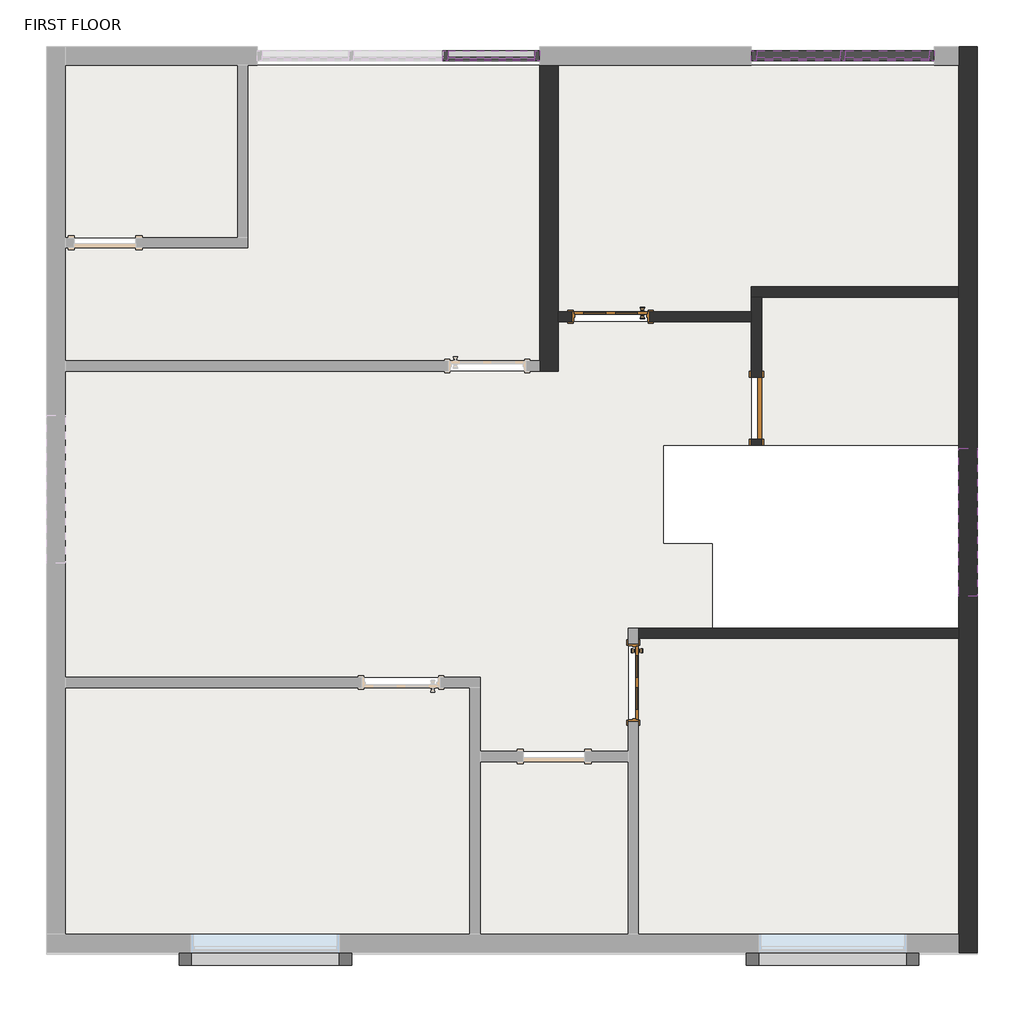
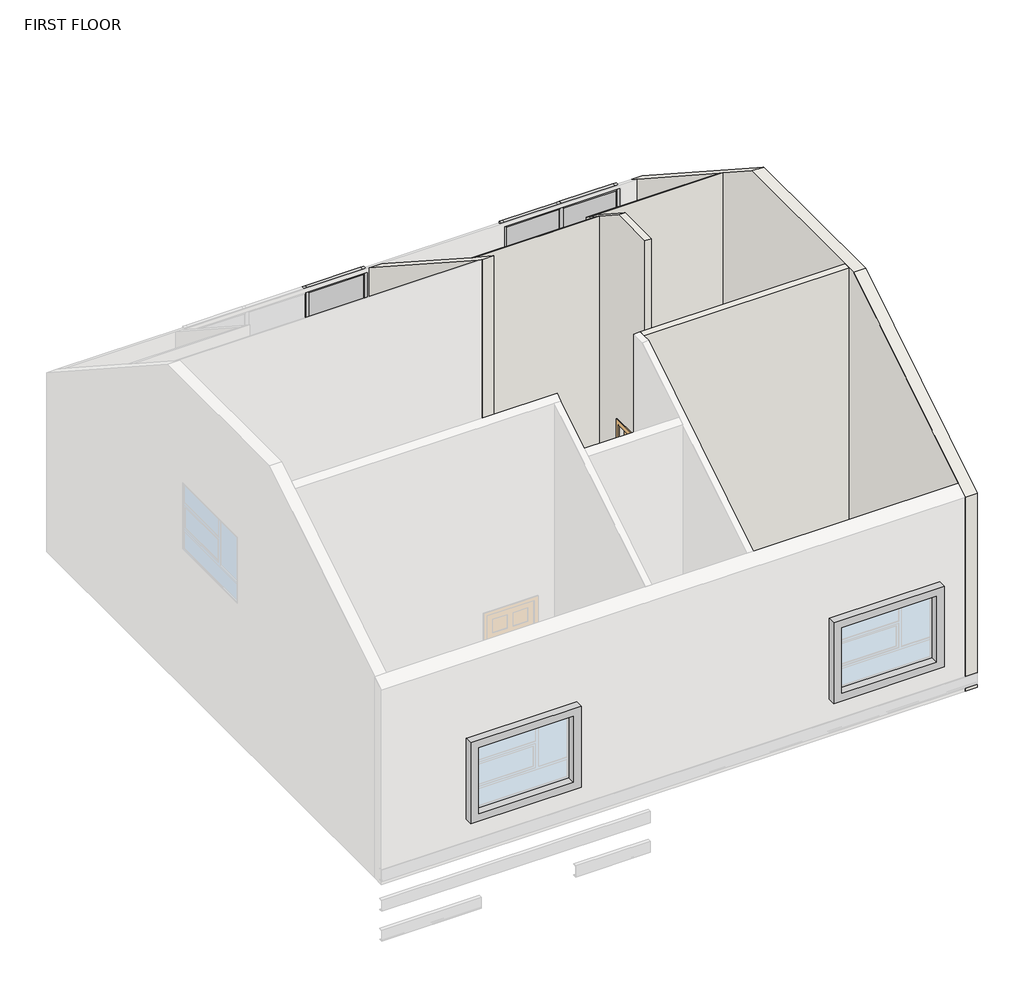
# One storey, part 2 of 2: 41 members, 14 plates, 6 walls, 3 doors, 2 proxies, 1 slab, 1 window.
"""IFC4 building model written with IfcOpenShell, lengths in millimetres."""

from ifc_helpers import new_model, si_unit, frame, origin, place, context, project, spatial, polyline, circle_curve, outline, extrude, faceted_brep, transform, mapped, element, save
from ifc_brep_helpers import plane_surface, cylinder_surface, revolved_surface, advanced_brep
from components import generic_models_4_generic_models_3_cea7143c, generic_models_5_generic_models_3_e9287e6f, door_03e3dfb5, door_c610b25b, door_1fe7f57d, member_693dcaa1, member_240932ed, member_6ef8dc49, member_6e77e263, member_4194b792, member_47bfaf8a, member_2b49869a, member_75074519, member_309cb93c, member_15f4dda0, member_2a4e9e33, system_panel_glazed_03e0ee66, system_panel_glazed_46ac4994, system_panel_glazed_368d4c1c, system_panel_glazed_c7bdd9bd, system_panel_glazed_ec73f643, system_panel_glazed_e581be51, system_panel_glazed_99f7726d, window_dd9b4f56

model = new_model("IFC4")

# Units and contexts
model_context = context("Model", 3, world=origin())
ifc_project = project(units=[si_unit("LENGTHUNIT", "METRE", prefix="MILLI")], contexts=[model_context])

# Site, building, storey
site = spatial("IfcSite", under=ifc_project)
building = spatial("IfcBuilding", under=site)
storey = spatial("IfcBuildingStorey", under=building, Name="FIRST FLOOR", Elevation=3352.8)

# Proxies
placement = place(None, origin())
generic_models_4_generic_models_3_shape = generic_models_4_generic_models_3_cea7143c(model_context)
element("IfcBuildingElementProxy", 1, Name="Generic Models 4 : Generic Models 3", ObjectType="Generic Models 4 : Generic Models 3", at=placement, inside=storey, context=model_context, shape_type="MappedRepresentation", body=[
    mapped(generic_models_4_generic_models_3_shape, transform((0.0, 0.0, 0.0), x_axis=(1.0, 0.0, 0.0), y_axis=(0.0, 1.0, 0.0), z_axis=(0.0, 0.0, 1.0))),
])
generic_models_5_generic_models_3_shape = generic_models_5_generic_models_3_e9287e6f(model_context)
element("IfcBuildingElementProxy", 2, Name="Generic Models 5 : Generic Models 3", ObjectType="Generic Models 5 : Generic Models 3", at=placement, inside=storey, context=model_context, shape_type="MappedRepresentation", body=[
    mapped(generic_models_5_generic_models_3_shape, transform((0.0, 0.0, 0.0), x_axis=(1.0, 0.0, 0.0), y_axis=(0.0, 1.0, 0.0), z_axis=(0.0, 0.0, 1.0))),
])

# Doors
door_shape = door_03e3dfb5(model_context)
element("IfcDoor", 3, ObjectType="Door-Interior-Single-6_Panel-Wood : 36\" x 84\"", at=placement, inside=storey, context=model_context, shape_type="MappedRepresentation", body=[
    mapped(door_shape, transform((1410.8421209, 890.2223211, 3352.8), x_axis=(0.0, -1.0, 0.0), y_axis=(1.0, 0.0, 0.0), z_axis=(0.0, 0.0, 1.0))),
])
door_2_shape = door_c610b25b(model_context)
element("IfcDoor", 4, ObjectType="Door-Interior-Single-6_Panel-Wood : 36\" x 84\"", at=placement, inside=storey, context=model_context, shape_type="MappedRepresentation", body=[
    mapped(door_2_shape, transform((1128.2671209, 5414.5973211, 3352.8), x_axis=(-1.0, 0.0, 0.0), y_axis=(0.0, -1.0, 0.0), z_axis=(0.0, 0.0, 1.0))),
])
door_3_shape = door_1fe7f57d(model_context)
element("IfcDoor", 5, ObjectType="Single-Flush : bathroom flush door 2' 6\" x 7'", at=placement, inside=storey, context=model_context, shape_type="MappedRepresentation", body=[
    mapped(door_3_shape, transform((2931.6671209, 4281.1223211, 3352.8), x_axis=(0.0, -1.0, 0.0), y_axis=(1.0, 0.0, 0.0), z_axis=(0.0, 0.0, 1.0))),
])

# Members
member_shape = member_693dcaa1(model_context)
element("IfcMember", 6, ObjectType="Rectangular Mullion : 2.5\" x 5\" rectangular", at=placement, inside=storey, context=model_context, shape_type="MappedRepresentation", body=[
    mapped(member_shape, transform((-880.4495459, 8637.2223211, 7085.0688597), x_axis=(0.0, 0.0, 1.0), y_axis=(0.0, 1.0, 0.0), z_axis=(-1.0, 0.0, 0.0))),
])
element("IfcMember", 7, ObjectType="Rectangular Mullion : 2.5\" x 5\" rectangular", at=placement, inside=storey, context=model_context, shape_type="MappedRepresentation", body=[
    mapped(member_shape, transform((188.4671209, 8637.2223211, 3352.8), x_axis=(0.0, 0.0, -1.0), y_axis=(0.0, 1.0, 0.0), z_axis=(1.0, 0.0, 0.0))),
])
member_2_shape = member_240932ed(model_context)
element("IfcMember", 8, ObjectType="Rectangular Mullion : 2.5\" x 5\" rectangular", at=placement, inside=storey, context=model_context, shape_type="MappedRepresentation", body=[
    mapped(member_2_shape, transform((-943.9495459, 8637.2223211, 3352.8), x_axis=(0.0, 0.0, -1.0), y_axis=(0.0, 1.0, 0.0), z_axis=(1.0, 0.0, 0.0))),
])
member_3_shape = member_6ef8dc49(model_context)
element("IfcMember", 9, ObjectType="Rectangular Mullion : 2.5\" x 5\" rectangular", at=placement, inside=storey, context=model_context, shape_type="MappedRepresentation", body=[
    mapped(member_3_shape, transform((2931.6671209, 8637.2223211, 7085.0688597), x_axis=(0.0, 0.0, 1.0), y_axis=(0.0, 1.0, 0.0), z_axis=(-1.0, 0.0, 0.0))),
])
element("IfcMember", 10, ObjectType="Rectangular Mullion : 2.5\" x 5\" rectangular", at=placement, inside=storey, context=model_context, shape_type="MappedRepresentation", body=[
    mapped(member_3_shape, transform((4030.2171209, 8637.2223211, 7085.0688597), x_axis=(0.0, 0.0, 1.0), y_axis=(0.0, 1.0, 0.0), z_axis=(-1.0, 0.0, 0.0))),
])
element("IfcMember", 11, ObjectType="Rectangular Mullion : 2.5\" x 5\" rectangular", at=placement, inside=storey, context=model_context, shape_type="MappedRepresentation", body=[
    mapped(member_3_shape, transform((5065.2671209, 8637.2223211, 3352.8), x_axis=(0.0, 0.0, -1.0), y_axis=(0.0, 1.0, 0.0), z_axis=(1.0, 0.0, 0.0))),
])
element("IfcMember", 12, ObjectType="Rectangular Mullion : 2.5\" x 5\" rectangular", at=placement, inside=storey, context=model_context, shape_type="MappedRepresentation", body=[
    mapped(member_3_shape, transform((3966.7171209, 8637.2223211, 3352.8), x_axis=(0.0, 0.0, -1.0), y_axis=(0.0, 1.0, 0.0), z_axis=(1.0, 0.0, 0.0))),
])
member_4_shape = member_6e77e263(model_context)
element("IfcMember", 13, ObjectType="Rectangular Mullion : 2.5\" x 5\" rectangular", at=placement, inside=storey, context=model_context, shape_type="MappedRepresentation", body=[
    mapped(member_4_shape, transform((-912.1995459, 8637.2223211, 3352.8), x_axis=(-1.0, 0.0, 0.0), y_axis=(0.0, 1.0, 0.0), z_axis=(0.0, 0.0, -1.0))),
])
element("IfcMember", 14, ObjectType="Rectangular Mullion : 2.5\" x 5\" rectangular", at=placement, inside=storey, context=model_context, shape_type="MappedRepresentation", body=[
    mapped(member_4_shape, transform((3998.4671209, 8637.2223211, 3352.8), x_axis=(-1.0, 0.0, 0.0), y_axis=(0.0, 1.0, 0.0), z_axis=(0.0, 0.0, -1.0))),
])
member_5_shape = member_4194b792(model_context)
element("IfcMember", 15, ObjectType="Rectangular Mullion : 2.5\" x 5\" rectangular", at=placement, inside=storey, context=model_context, shape_type="MappedRepresentation", body=[
    mapped(member_5_shape, transform((-880.4495459, 8637.2223211, 3962.4), x_axis=(0.0, 0.0, 1.0), y_axis=(0.0, 1.0, 0.0), z_axis=(-1.0, 0.0, 0.0))),
])
element("IfcMember", 16, ObjectType="Rectangular Mullion : 2.5\" x 5\" rectangular", at=placement, inside=storey, context=model_context, shape_type="MappedRepresentation", body=[
    mapped(member_5_shape, transform((-880.4495459, 8637.2223211, 5181.6), x_axis=(0.0, 0.0, 1.0), y_axis=(0.0, 1.0, 0.0), z_axis=(-1.0, 0.0, 0.0))),
])
element("IfcMember", 17, ObjectType="Rectangular Mullion : 2.5\" x 5\" rectangular", at=placement, inside=storey, context=model_context, shape_type="MappedRepresentation", body=[
    mapped(member_5_shape, transform((-880.4495459, 8637.2223211, 5791.2), x_axis=(0.0, 0.0, 1.0), y_axis=(0.0, 1.0, 0.0), z_axis=(-1.0, 0.0, 0.0))),
])
member_6_shape = member_47bfaf8a(model_context)
element("IfcMember", 18, ObjectType="Rectangular Mullion : 2.5\" x 5\" rectangular", at=placement, inside=storey, context=model_context, shape_type="MappedRepresentation", body=[
    mapped(member_6_shape, transform((2868.1671209, 8637.2223211, 3352.8), x_axis=(-1.0, 0.0, 0.0), y_axis=(0.0, 1.0, 0.0), z_axis=(0.0, 0.0, -1.0))),
])
element("IfcMember", 19, ObjectType="Rectangular Mullion : 2.5\" x 5\" rectangular", at=placement, inside=storey, context=model_context, shape_type="MappedRepresentation", body=[
    mapped(member_6_shape, transform((251.9671209, 8637.2223211, 3962.4), x_axis=(1.0, 0.0, 0.0), y_axis=(0.0, 1.0, 0.0), z_axis=(0.0, 0.0, 1.0))),
])
element("IfcMember", 20, ObjectType="Rectangular Mullion : 2.5\" x 5\" rectangular", at=placement, inside=storey, context=model_context, shape_type="MappedRepresentation", body=[
    mapped(member_6_shape, transform((5128.7671209, 8637.2223211, 3962.4), x_axis=(1.0, 0.0, 0.0), y_axis=(0.0, 1.0, 0.0), z_axis=(0.0, 0.0, 1.0))),
])
member_7_shape = member_2b49869a(model_context)
element("IfcMember", 21, ObjectType="Rectangular Mullion : 2.5\" x 5\" rectangular", at=placement, inside=storey, context=model_context, shape_type="MappedRepresentation", body=[
    mapped(member_7_shape, transform((-912.1995459, 8637.2223211, 3962.4), x_axis=(-1.0, 0.0, 0.0), y_axis=(0.0, 1.0, 0.0), z_axis=(0.0, 0.0, -1.0))),
])
member_8_shape = member_75074519(model_context)
element("IfcMember", 22, ObjectType="Rectangular Mullion : 2.5\" x 5\" rectangular", at=placement, inside=storey, context=model_context, shape_type="MappedRepresentation", body=[
    mapped(member_8_shape, transform((251.9671209, 8637.2223211, 5181.6), x_axis=(1.0, 0.0, 0.0), y_axis=(0.0, 1.0, 0.0), z_axis=(0.0, 0.0, 1.0))),
])
member_9_shape = member_309cb93c(model_context)
element("IfcMember", 23, ObjectType="Rectangular Mullion : 2.5\" x 5\" rectangular", at=placement, inside=storey, context=model_context, shape_type="MappedRepresentation", body=[
    mapped(member_9_shape, transform((4030.2171209, 8637.2223211, 5791.2), x_axis=(0.0, 0.0, 1.0), y_axis=(0.0, 1.0, 0.0), z_axis=(-1.0, 0.0, 0.0))),
])
element("IfcMember", 24, ObjectType="Rectangular Mullion : 2.5\" x 5\" rectangular", at=placement, inside=storey, context=model_context, shape_type="MappedRepresentation", body=[
    mapped(member_9_shape, transform((2931.6671209, 8637.2223211, 5791.2), x_axis=(0.0, 0.0, 1.0), y_axis=(0.0, 1.0, 0.0), z_axis=(-1.0, 0.0, 0.0))),
])
element("IfcMember", 25, ObjectType="Rectangular Mullion : 2.5\" x 5\" rectangular", at=placement, inside=storey, context=model_context, shape_type="MappedRepresentation", body=[
    mapped(member_9_shape, transform((4030.2171209, 8637.2223211, 5181.6), x_axis=(0.0, 0.0, 1.0), y_axis=(0.0, 1.0, 0.0), z_axis=(-1.0, 0.0, 0.0))),
])
element("IfcMember", 26, ObjectType="Rectangular Mullion : 2.5\" x 5\" rectangular", at=placement, inside=storey, context=model_context, shape_type="MappedRepresentation", body=[
    mapped(member_9_shape, transform((2931.6671209, 8637.2223211, 5181.6), x_axis=(0.0, 0.0, 1.0), y_axis=(0.0, 1.0, 0.0), z_axis=(-1.0, 0.0, 0.0))),
])
element("IfcMember", 27, ObjectType="Rectangular Mullion : 2.5\" x 5\" rectangular", at=placement, inside=storey, context=model_context, shape_type="MappedRepresentation", body=[
    mapped(member_9_shape, transform((4030.2171209, 8637.2223211, 4572.0), x_axis=(0.0, 0.0, 1.0), y_axis=(0.0, 1.0, 0.0), z_axis=(-1.0, 0.0, 0.0))),
])
element("IfcMember", 28, ObjectType="Rectangular Mullion : 2.5\" x 5\" rectangular", at=placement, inside=storey, context=model_context, shape_type="MappedRepresentation", body=[
    mapped(member_9_shape, transform((2931.6671209, 8637.2223211, 4572.0), x_axis=(0.0, 0.0, 1.0), y_axis=(0.0, 1.0, 0.0), z_axis=(-1.0, 0.0, 0.0))),
])
element("IfcMember", 29, ObjectType="Rectangular Mullion : 2.5\" x 5\" rectangular", at=placement, inside=storey, context=model_context, shape_type="MappedRepresentation", body=[
    mapped(member_9_shape, transform((4030.2171209, 8637.2223211, 3962.4), x_axis=(0.0, 0.0, 1.0), y_axis=(0.0, 1.0, 0.0), z_axis=(-1.0, 0.0, 0.0))),
])
element("IfcMember", 30, ObjectType="Rectangular Mullion : 2.5\" x 5\" rectangular", at=placement, inside=storey, context=model_context, shape_type="MappedRepresentation", body=[
    mapped(member_9_shape, transform((2931.6671209, 8637.2223211, 3962.4), x_axis=(0.0, 0.0, 1.0), y_axis=(0.0, 1.0, 0.0), z_axis=(-1.0, 0.0, 0.0))),
])
element("IfcMember", 31, ObjectType="Rectangular Mullion : 2.5\" x 5\" rectangular", at=placement, inside=storey, context=model_context, shape_type="MappedRepresentation", body=[
    mapped(member_4_shape, transform((-912.1995459, 8637.2223211, 5181.6), x_axis=(-1.0, 0.0, 0.0), y_axis=(0.0, 1.0, 0.0), z_axis=(0.0, 0.0, -1.0))),
])
element("IfcMember", 32, ObjectType="Rectangular Mullion : 2.5\" x 5\" rectangular", at=placement, inside=storey, context=model_context, shape_type="MappedRepresentation", body=[
    mapped(member_4_shape, transform((3998.4671209, 8637.2223211, 5181.6), x_axis=(-1.0, 0.0, 0.0), y_axis=(0.0, 1.0, 0.0), z_axis=(0.0, 0.0, -1.0))),
])
element("IfcMember", 33, ObjectType="Rectangular Mullion : 2.5\" x 5\" rectangular", at=placement, inside=storey, context=model_context, shape_type="MappedRepresentation", body=[
    mapped(member_4_shape, transform((3998.4671209, 8637.2223211, 4572.0), x_axis=(-1.0, 0.0, 0.0), y_axis=(0.0, 1.0, 0.0), z_axis=(0.0, 0.0, -1.0))),
])
element("IfcMember", 34, ObjectType="Rectangular Mullion : 2.5\" x 5\" rectangular", at=placement, inside=storey, context=model_context, shape_type="MappedRepresentation", body=[
    mapped(member_4_shape, transform((3998.4671209, 8637.2223211, 3962.4), x_axis=(-1.0, 0.0, 0.0), y_axis=(0.0, 1.0, 0.0), z_axis=(0.0, 0.0, -1.0))),
])
element("IfcMember", 35, ObjectType="Rectangular Mullion : 2.5\" x 5\" rectangular", at=placement, inside=storey, context=model_context, shape_type="MappedRepresentation", body=[
    mapped(member_6_shape, transform((5128.7671209, 8637.2223211, 5791.2), x_axis=(1.0, 0.0, 0.0), y_axis=(0.0, 1.0, 0.0), z_axis=(0.0, 0.0, 1.0))),
])
element("IfcMember", 36, ObjectType="Rectangular Mullion : 2.5\" x 5\" rectangular", at=placement, inside=storey, context=model_context, shape_type="MappedRepresentation", body=[
    mapped(member_6_shape, transform((5128.7671209, 8637.2223211, 5181.6), x_axis=(1.0, 0.0, 0.0), y_axis=(0.0, 1.0, 0.0), z_axis=(0.0, 0.0, 1.0))),
])
element("IfcMember", 37, ObjectType="Rectangular Mullion : 2.5\" x 5\" rectangular", at=placement, inside=storey, context=model_context, shape_type="MappedRepresentation", body=[
    mapped(member_6_shape, transform((5128.7671209, 8637.2223211, 4572.0), x_axis=(1.0, 0.0, 0.0), y_axis=(0.0, 1.0, 0.0), z_axis=(0.0, 0.0, 1.0))),
])
element("IfcMember", 38, ObjectType="Rectangular Mullion : 2.5\" x 5\" rectangular", at=placement, inside=storey, context=model_context, shape_type="MappedRepresentation", body=[
    mapped(member_6_shape, transform((251.9671209, 8637.2223211, 5791.2), x_axis=(1.0, 0.0, 0.0), y_axis=(0.0, 1.0, 0.0), z_axis=(0.0, 0.0, 1.0))),
])
element("IfcMember", 39, ObjectType="Rectangular Mullion : 2.5\" x 5\" rectangular", at=placement, inside=storey, context=model_context, shape_type="MappedRepresentation", body=[
    mapped(member_6_shape, transform((2868.1671209, 8637.2223211, 5181.6), x_axis=(-1.0, 0.0, 0.0), y_axis=(0.0, 1.0, 0.0), z_axis=(0.0, 0.0, -1.0))),
])
element("IfcMember", 40, ObjectType="Rectangular Mullion : 2.5\" x 5\" rectangular", at=placement, inside=storey, context=model_context, shape_type="MappedRepresentation", body=[
    mapped(member_6_shape, transform((2868.1671209, 8637.2223211, 4572.0), x_axis=(-1.0, 0.0, 0.0), y_axis=(0.0, 1.0, 0.0), z_axis=(0.0, 0.0, -1.0))),
])
element("IfcMember", 41, ObjectType="Rectangular Mullion : 2.5\" x 5\" rectangular", at=placement, inside=storey, context=model_context, shape_type="MappedRepresentation", body=[
    mapped(member_6_shape, transform((2868.1671209, 8637.2223211, 3962.4), x_axis=(-1.0, 0.0, 0.0), y_axis=(0.0, 1.0, 0.0), z_axis=(0.0, 0.0, -1.0))),
])
member_10_shape = member_15f4dda0(model_context)
element("IfcMember", 42, ObjectType="Rectangular Mullion : 2.5\" x 5\" rectangular", at=placement, inside=storey, context=model_context, shape_type="MappedRepresentation", body=[
    mapped(member_10_shape, transform((3998.4671209, 8637.2223211, 5791.2), x_axis=(-1.0, 0.0, 0.0), y_axis=(0.0, 1.0, 0.0), z_axis=(0.0, 0.0, -1.0))),
])
element("IfcMember", 43, ObjectType="Rectangular Mullion : 2.5\" x 5\" rectangular", at=placement, inside=storey, context=model_context, shape_type="MappedRepresentation", body=[
    mapped(member_10_shape, transform((-912.1995459, 8637.2223211, 5791.2), x_axis=(-1.0, 0.0, 0.0), y_axis=(0.0, 1.0, 0.0), z_axis=(0.0, 0.0, -1.0))),
])
member_11_shape = member_2a4e9e33(model_context)
element("IfcMember", 44, ObjectType="Rectangular Mullion : 2.5\" x 5\" rectangular", at=placement, inside=storey, context=model_context, shape_type="MappedRepresentation", body=[
    mapped(member_11_shape, transform((251.9671209, 8637.2223211, 7085.0688597), x_axis=(1.0, 0.0, 0.0), y_axis=(0.0, 1.0, 0.0), z_axis=(0.0, 0.0, 1.0))),
])
element("IfcMember", 45, ObjectType="Rectangular Mullion : 2.5\" x 5\" rectangular", at=placement, inside=storey, context=model_context, shape_type="MappedRepresentation", body=[
    mapped(member_11_shape, transform((5128.7671209, 8637.2223211, 7085.0688597), x_axis=(1.0, 0.0, 0.0), y_axis=(0.0, 1.0, 0.0), z_axis=(0.0, 0.0, 1.0))),
])
element("IfcMember", 46, ObjectType="Rectangular Mullion : 2.5\" x 5\" rectangular", at=placement, inside=storey, context=model_context, shape_type="MappedRepresentation", body=[
    mapped(member_11_shape, transform((2868.1671209, 8637.2223211, 5791.2), x_axis=(-1.0, 0.0, 0.0), y_axis=(0.0, 1.0, 0.0), z_axis=(0.0, 0.0, -1.0))),
])

# Plates
system_panel_glazed_shape = system_panel_glazed_03e0ee66(model_context)
element("IfcPlate", 47, ObjectType="System Panel : Glazed", at=placement, inside=storey, context=model_context, shape_type="MappedRepresentation", body=[
    mapped(system_panel_glazed_shape, transform((-345.9912125, 8637.2223211, 3416.3), x_axis=(-1.0, 0.0, 0.0), y_axis=(0.0, -1.0, 0.0), z_axis=(0.0, 0.0, 1.0))),
])
system_panel_glazed_2_shape = system_panel_glazed_46ac4994(model_context)
element("IfcPlate", 48, ObjectType="System Panel : Glazed", at=placement, inside=storey, context=model_context, shape_type="MappedRepresentation", body=[
    mapped(system_panel_glazed_2_shape, transform((-345.9912125, 8637.2223211, 3994.15), x_axis=(-1.0, 0.0, 0.0), y_axis=(0.0, -1.0, 0.0), z_axis=(0.0, 0.0, 1.0))),
])
system_panel_glazed_3_shape = system_panel_glazed_368d4c1c(model_context)
element("IfcPlate", 49, ObjectType="System Panel : Glazed", at=placement, inside=storey, context=model_context, shape_type="MappedRepresentation", body=[
    mapped(system_panel_glazed_3_shape, transform((4547.7421209, 8637.2223211, 3416.3), x_axis=(-1.0, 0.0, 0.0), y_axis=(0.0, -1.0, 0.0), z_axis=(0.0, 0.0, 1.0))),
])
element("IfcPlate", 50, ObjectType="System Panel : Glazed", at=placement, inside=storey, context=model_context, shape_type="MappedRepresentation", body=[
    mapped(system_panel_glazed_3_shape, transform((3449.1921209, 8637.2223211, 3416.3), x_axis=(-1.0, 0.0, 0.0), y_axis=(0.0, -1.0, 0.0), z_axis=(0.0, 0.0, 1.0))),
])
system_panel_glazed_4_shape = system_panel_glazed_c7bdd9bd(model_context)
element("IfcPlate", 51, ObjectType="System Panel : Glazed", at=placement, inside=storey, context=model_context, shape_type="MappedRepresentation", body=[
    mapped(system_panel_glazed_4_shape, transform((4547.7421209, 8637.2223211, 5213.35), x_axis=(-1.0, 0.0, 0.0), y_axis=(0.0, -1.0, 0.0), z_axis=(0.0, 0.0, 1.0))),
])
element("IfcPlate", 52, ObjectType="System Panel : Glazed", at=placement, inside=storey, context=model_context, shape_type="MappedRepresentation", body=[
    mapped(system_panel_glazed_4_shape, transform((3449.1921209, 8637.2223211, 5213.35), x_axis=(-1.0, 0.0, 0.0), y_axis=(0.0, -1.0, 0.0), z_axis=(0.0, 0.0, 1.0))),
])
element("IfcPlate", 53, ObjectType="System Panel : Glazed", at=placement, inside=storey, context=model_context, shape_type="MappedRepresentation", body=[
    mapped(system_panel_glazed_4_shape, transform((4547.7421209, 8637.2223211, 4603.75), x_axis=(-1.0, 0.0, 0.0), y_axis=(0.0, -1.0, 0.0), z_axis=(0.0, 0.0, 1.0))),
])
element("IfcPlate", 54, ObjectType="System Panel : Glazed", at=placement, inside=storey, context=model_context, shape_type="MappedRepresentation", body=[
    mapped(system_panel_glazed_4_shape, transform((3449.1921209, 8637.2223211, 4603.75), x_axis=(-1.0, 0.0, 0.0), y_axis=(0.0, -1.0, 0.0), z_axis=(0.0, 0.0, 1.0))),
])
element("IfcPlate", 55, ObjectType="System Panel : Glazed", at=placement, inside=storey, context=model_context, shape_type="MappedRepresentation", body=[
    mapped(system_panel_glazed_4_shape, transform((4547.7421209, 8637.2223211, 3994.15), x_axis=(-1.0, 0.0, 0.0), y_axis=(0.0, -1.0, 0.0), z_axis=(0.0, 0.0, 1.0))),
])
element("IfcPlate", 56, ObjectType="System Panel : Glazed", at=placement, inside=storey, context=model_context, shape_type="MappedRepresentation", body=[
    mapped(system_panel_glazed_4_shape, transform((3449.1921209, 8637.2223211, 3994.15), x_axis=(-1.0, 0.0, 0.0), y_axis=(0.0, -1.0, 0.0), z_axis=(0.0, 0.0, 1.0))),
])
system_panel_glazed_5_shape = system_panel_glazed_ec73f643(model_context)
element("IfcPlate", 57, ObjectType="System Panel : Glazed", at=placement, inside=storey, context=model_context, shape_type="MappedRepresentation", body=[
    mapped(system_panel_glazed_5_shape, transform((4547.7421209, 8637.2223211, 5822.95), x_axis=(-1.0, 0.0, 0.0), y_axis=(0.0, -1.0, 0.0), z_axis=(0.0, 0.0, 1.0))),
])
element("IfcPlate", 58, ObjectType="System Panel : Glazed", at=placement, inside=storey, context=model_context, shape_type="MappedRepresentation", body=[
    mapped(system_panel_glazed_5_shape, transform((3449.1921209, 8637.2223211, 5822.95), x_axis=(-1.0, 0.0, 0.0), y_axis=(0.0, -1.0, 0.0), z_axis=(0.0, 0.0, 1.0))),
])
system_panel_glazed_6_shape = system_panel_glazed_e581be51(model_context)
element("IfcPlate", 59, ObjectType="System Panel : Glazed", at=placement, inside=storey, context=model_context, shape_type="MappedRepresentation", body=[
    mapped(system_panel_glazed_6_shape, transform((-345.9912125, 8637.2223211, 5213.35), x_axis=(-1.0, 0.0, 0.0), y_axis=(0.0, -1.0, 0.0), z_axis=(0.0, 0.0, 1.0))),
])
system_panel_glazed_7_shape = system_panel_glazed_99f7726d(model_context)
element("IfcPlate", 60, ObjectType="System Panel : Glazed", at=placement, inside=storey, context=model_context, shape_type="MappedRepresentation", body=[
    mapped(system_panel_glazed_7_shape, transform((-345.9912125, 8637.2223211, 5822.95), x_axis=(-1.0, 0.0, 0.0), y_axis=(0.0, -1.0, 0.0), z_axis=(0.0, 0.0, 1.0))),
])

# Slab
element("IfcSlab", 61, ObjectType="marble flooring 1' 2", at=placement, inside=storey, context=model_context, shape_type="SweptSolid", body=[
    extrude(outline(polyline([(-3481.8328791, 8522.9223211), (-3481.8328791, 6389.3223211), (-5615.4328791, 6389.3223211), (-5615.4328791, 8522.9223211), (-3481.8328791, 8522.9223211)])), frame((0.0, 0.0, 3200.4), z_axis=(0.0, 0.0, 1.0), x_axis=(1.0, 0.0, 0.0)), (0.0, 0.0, 1.0), 152.4),
    extrude(outline(polyline([(5433.5671209, 5652.7223211), (5433.5671209, 3823.9223211), (2995.1671209, 3823.9223211), (2995.1671209, 5652.7223211), (5433.5671209, 5652.7223211)])), frame((0.0, 0.0, 3200.4), z_axis=(0.0, 0.0, 1.0), x_axis=(1.0, 0.0, 0.0)), (0.0, 0.0, 1.0), 152.4),
    extrude(outline(polyline([(-611.6328791, 826.7223211), (-611.6328791, -2221.2776789), (-5615.4328791, -2221.2776789), (-5615.4328791, 826.7223211), (-611.6328791, 826.7223211)])), frame((0.0, 0.0, 3200.4), z_axis=(0.0, 0.0, 1.0), x_axis=(1.0, 0.0, 0.0)), (0.0, 0.0, 1.0), 152.4),
    extrude(outline(polyline([(5433.5671209, 1436.3223211), (5433.5671209, -2221.2776789), (1471.1671209, -2221.2776789), (1471.1671209, 1436.3223211), (5433.5671209, 1436.3223211)])), frame((0.0, 0.0, 3200.4), z_axis=(0.0, 0.0, 1.0), x_axis=(1.0, 0.0, 0.0)), (0.0, 0.0, 1.0), 152.4),
    extrude(outline(polyline([(-5615.4328791, 6262.3223211), (-3354.8328791, 6262.3223211), (-3354.8328791, 8522.9223211), (251.9671209, 8522.9223211), (251.9671209, 4865.3223211), (-5615.4328791, 4865.3223211), (-5615.4328791, 6262.3223211)])), frame((0.0, 0.0, 3200.4), z_axis=(0.0, 0.0, 1.0), x_axis=(1.0, 0.0, 0.0)), (0.0, 0.0, 1.0), 152.4),
    extrude(outline(polyline([(5433.5671209, 8522.9223211), (5433.5671209, 5779.7223211), (2868.1671209, 5779.7223211), (2868.1671209, 5474.9223211), (480.5671209, 5474.9223211), (480.5671209, 8522.9223211), (5433.5671209, 8522.9223211)])), frame((0.0, 0.0, 3200.4), z_axis=(0.0, 0.0, 1.0), x_axis=(1.0, 0.0, 0.0)), (0.0, 0.0, 1.0), 152.4),
    extrude(outline(polyline([(1344.1671209, -2221.2776789), (-484.6328791, -2221.2776789), (-484.6328791, -87.6776789), (1344.1671209, -87.6776789), (1344.1671209, -2221.2776789)])), frame((0.0, 0.0, 3200.4), z_axis=(0.0, 0.0, 1.0), x_axis=(1.0, 0.0, 0.0)), (0.0, 0.0, 1.0), 152.4),
    extrude(outline(polyline([(-5615.4328791, 953.7223211), (-5615.4328791, 4738.3223211), (480.5671209, 4738.3223211), (480.5671209, 5347.9223211), (2868.1671209, 5347.9223211), (2868.1671209, 3823.9223211), (1775.9671209, 3823.9223211), (1775.9671209, 2604.7223211), (2385.5671209, 2604.7223211), (2385.5671209, 1563.3223211), (1344.1671209, 1563.3223211), (1344.1671209, 39.3223211), (-484.6328791, 39.3223211), (-484.6328791, 953.7223211), (-5615.4328791, 953.7223211)])), frame((0.0, 0.0, 3200.4), z_axis=(0.0, 0.0, 1.0), x_axis=(1.0, 0.0, 0.0)), (0.0, 0.0, 1.0), 152.4),
])

# Walls
element("IfcWall", 62, ObjectType="INNER WALL 5\"", at=placement, inside=storey, context=model_context, shape_type="Brep", body=[
    faceted_brep([(480.5671209, 5347.9223211, 9221.165256), (480.5671209, 5347.9223211, 3352.8), (645.6671209, 5347.9223211, 3352.8), (645.6671209, 5347.9223211, 5511.8), (1610.8671209, 5347.9223211, 5511.8), (1610.8671209, 5347.9223211, 3352.8), (2868.1671209, 5347.9223211, 3352.8), (2868.1671209, 5347.9223211, 9221.165256), (480.5671209, 5474.9223211, 3352.8), (480.5671209, 5474.9223211, 9138.6904917), (2868.1671209, 5474.9223211, 9138.6904917), (2868.1671209, 5474.9223211, 3352.8), (1610.8671209, 5474.9223211, 3352.8), (1610.8671209, 5474.9223211, 5511.8), (645.6671209, 5474.9223211, 5511.8), (645.6671209, 5474.9223211, 3352.8)], [[[0, 1, 2, 3, 4, 5, 6, 7]], [[8, 9, 10, 11, 12, 13, 14, 15]], [[1, 8, 15, 2]], [[11, 6, 5, 12]], [[1, 0, 9, 8]], [[7, 6, 11, 10]], [[14, 3, 2, 15]], [[3, 14, 13, 4]], [[4, 13, 12, 5]], [[0, 7, 10, 9]]]),
])
element("IfcWall", 63, ObjectType="INNER WALL 5\"", at=placement, inside=storey, context=model_context, shape_type="Brep", body=[
    faceted_brep([(5433.5671209, 5779.7223211, 3352.8), (2868.1671209, 5779.7223211, 3352.8), (2868.1671209, 5779.7223211, 8940.7510573), (5433.5671209, 5779.7223211, 8940.7510573), (5433.5671209, 5652.7223211, 3352.8), (5433.5671209, 5652.7223211, 9023.2258216), (2995.1671209, 5652.7223211, 9023.2258216), (2868.1671209, 5652.7223211, 9023.2258216), (2868.1671209, 5652.7223211, 3352.8), (2995.1671209, 5652.7223211, 3352.8)], [[[0, 1, 2, 3]], [[4, 5, 6, 7, 8, 9]], [[1, 0, 4, 9, 8]], [[0, 3, 5, 4]], [[2, 1, 8, 7]], [[3, 2, 7, 6, 5]]]),
])
element("IfcWall", 64, ObjectType="INNER WALL 5\"", at=placement, inside=storey, context=model_context, shape_type="Brep", body=[
    faceted_brep([(2868.1671209, 3900.1223211, 5384.8), (2868.1671209, 3900.1223211, 3352.8), (2868.1671209, 3823.9223211, 3352.8), (2868.1671209, 3823.9223211, 9646.3602906), (2868.1671209, 4693.1793845, 9646.3602906), (2868.1671209, 5347.9223211, 9221.165256), (2868.1671209, 5474.9223211, 9138.6904917), (2868.1671209, 5652.7223211, 9023.2258216), (2868.1671209, 5652.7223211, 3352.8), (2868.1671209, 5474.9223211, 3352.8), (2868.1671209, 5347.9223211, 3352.8), (2868.1671209, 4662.1223211, 3352.8), (2868.1671209, 4662.1223211, 5384.8), (2995.1671209, 3823.9223211, 3352.8), (2995.1671209, 3900.1223211, 3352.8), (2995.1671209, 3900.1223211, 5384.8), (2995.1671209, 4662.1223211, 5384.8), (2995.1671209, 4662.1223211, 3352.8), (2995.1671209, 5652.7223211, 3352.8), (2995.1671209, 5652.7223211, 9023.2258216), (2995.1671209, 4693.1793845, 9646.3602906), (2995.1671209, 3823.9223211, 9646.3602906)], [[[0, 1, 2, 3, 4, 5, 6, 7, 8, 9, 10, 11, 12]], [[13, 14, 15, 16, 17, 18, 19, 20, 21]], [[2, 1, 14, 13]], [[11, 10, 9, 8, 18, 17]], [[3, 2, 13, 21]], [[8, 7, 19, 18]], [[15, 14, 1, 0]], [[16, 15, 0, 12]], [[17, 16, 12, 11]], [[7, 6, 5, 4, 20, 19]], [[4, 3, 21, 20]]]),
])
element("IfcWall", 65, ObjectType="INNER WALL 5\"", at=placement, inside=storey, context=model_context, shape_type="SweptSolid", body=[
    extrude(outline(polyline([(5433.5671209, 1436.3223211), (1471.1671209, 1436.3223211), (1471.1671209, 1563.3223211), (5433.5671209, 1563.3223211), (5433.5671209, 1436.3223211)])), frame((0.0, 0.0, 3352.8), z_axis=(0.0, 0.0, 1.0), x_axis=(1.0, 0.0, 0.0)), (0.0, 0.0, 1.0), 6293.5602906),
])
element("IfcWall", 66, ObjectType="OUTER WALL 9\"", at=placement, inside=storey, context=model_context, shape_type="AdvancedBrep", body=[
    advanced_brep(
    [(5433.5671209, 8751.5223211, 3352.8), (5433.5671209, 8522.9223211, 3352.8), (5433.5671209, 5779.7223211, 3352.8), (5433.5671209, 5652.7223211, 3352.8), (5433.5671209, 1563.3223211, 3352.8), (5433.5671209, 1436.3223211, 3352.8), (5433.5671209, -2221.2776789, 3352.8), (5433.5671209, -2449.8776789, 3352.8), (5433.5671209, -2449.8776789, 3424.313469), (5433.5671209, -2401.5160789, 3424.313469), (5433.5671209, -2401.5160789, 3425.6931449), (5433.5671209, -2405.8988881, 3430.8668793), (5433.5671209, -2429.5195789, 3434.803669), (5433.5671209, -2448.7574605, 3438.009989), (5433.5671209, -2449.8776789, 3438.260359), (5433.5671209, -2449.8776789, 3638.9665791), (5433.5671209, -2448.7574605, 3639.216949), (5433.5671209, -2429.5195789, 3642.423269), (5433.5671209, -2405.8988881, 3646.3600587), (5433.5671209, -2401.5160789, 3651.5337932), (5433.5671209, -2401.5160789, 3652.913469), (5433.5671209, -2449.8776789, 3652.913469), (5433.5671209, -2449.8776789, 7317.6596789), (5433.5671209, -2221.2776789, 7460.5048127), (5433.5671209, 1276.8223179, 9646.3602906), (5433.5671209, 1436.3223211, 9646.3602906), (5433.5671209, 1563.3223211, 9646.3602906), (5433.5671209, 4693.1793845, 9646.3602906), (5433.5671209, 5652.7223211, 9023.2258216), (5433.5671209, 5779.7223211, 8940.7510573), (5433.5671209, 8522.9223211, 7159.2961476), (5433.5671209, 8751.5223211, 7010.8415718), (5433.5671209, 1957.0223211, 7735.9043115), (5433.5671209, 1957.0223211, 6389.7043115), (5433.5671209, 3785.8223211, 6389.7043115), (5433.5671209, 3785.8223211, 7735.9043115), (5662.1671209, -2449.8776789, 3352.8), (5662.1671209, 8751.5223211, 3352.8), (5662.1671209, 8751.5223211, 7010.8415718), (5662.1671209, 4693.1793845, 9646.3602906), (5662.1671209, 1276.8223179, 9646.3602906), (5662.1671209, -2449.8776789, 7317.6596789), (5662.1671209, -2449.8776789, 3652.913469), (5662.1671209, -2401.5160789, 3652.913469), (5662.1671209, -2401.5160789, 3651.5337932), (5662.1671209, -2405.8988881, 3646.3600587), (5662.1671209, -2429.5195789, 3642.423269), (5662.1671209, -2448.7574605, 3639.216949), (5662.1671209, -2449.8776789, 3638.9665791), (5662.1671209, -2449.8776789, 3438.260359), (5662.1671209, -2448.7574605, 3438.009989), (5662.1671209, -2429.5195789, 3434.803669), (5662.1671209, -2405.8988881, 3430.8668793), (5662.1671209, -2401.5160789, 3425.6931449), (5662.1671209, -2401.5160789, 3424.313469), (5662.1671209, -2449.8776789, 3424.313469), (5662.1671209, 1957.0223211, 6389.7043115), (5662.1671209, 1957.0223211, 7735.9043115), (5662.1671209, 3785.8223211, 7735.9043115), (5662.1671209, 3785.8223211, 6389.7043115)],
    [
        (0, 1),
        (1, 2),
        (2, 3),
        (3, 4),
        (4, 5),
        (5, 6),
        (6, 7),
        (7, 8),
        (8, 9),
        (9, 10),
        (10, 11, circle_curve(frame((5433.5671209, -2406.7611789, 3425.6931449), z_axis=(1.0, 0.0, 0.0), x_axis=(0.0, 1.0, 0.0)), 5.2451)),
        (11, 12),
        (12, 13),
        (13, 14, circle_curve(frame((5433.5671209, -2447.0328789, 3448.357458), z_axis=(-1.0, 0.0, 0.0), x_axis=(0.0, 1.0, 0.0)), 10.4902)),
        (14, 15),
        (15, 16, circle_curve(frame((5433.5671209, -2447.0328789, 3628.86948), z_axis=(-1.0, 0.0, 0.0), x_axis=(0.0, 1.0, 0.0)), 10.4902)),
        (16, 17),
        (17, 18),
        (18, 19, circle_curve(frame((5433.5671209, -2406.7611789, 3651.5337932), z_axis=(1.0, 0.0, 0.0), x_axis=(0.0, 1.0, 0.0)), 5.2451)),
        (19, 20),
        (20, 21),
        (21, 22),
        (22, 23),
        (23, 24),
        (24, 25),
        (25, 26),
        (26, 27),
        (27, 28),
        (28, 29),
        (29, 30),
        (30, 31),
        (31, 0),
        (32, 33),
        (33, 34),
        (34, 35),
        (35, 32),
        (36, 37),
        (37, 38),
        (38, 39),
        (39, 40),
        (40, 41),
        (41, 42),
        (42, 43),
        (43, 44),
        (44, 45, circle_curve(frame((5662.1671209, -2406.7611789, 3651.5337932), z_axis=(-1.0, 0.0, 0.0), x_axis=(0.0, 1.0, 0.0)), 5.2451)),
        (45, 46),
        (46, 47),
        (47, 48, circle_curve(frame((5662.1671209, -2447.0328789, 3628.86948), z_axis=(1.0, 0.0, 0.0), x_axis=(0.0, 1.0, 0.0)), 10.4902)),
        (48, 49),
        (49, 50, circle_curve(frame((5662.1671209, -2447.0328789, 3448.357458), z_axis=(1.0, 0.0, 0.0), x_axis=(0.0, 1.0, 0.0)), 10.4902)),
        (50, 51),
        (51, 52),
        (52, 53, circle_curve(frame((5662.1671209, -2406.7611789, 3425.6931449), z_axis=(-1.0, 0.0, 0.0), x_axis=(0.0, 1.0, 0.0)), 5.2451)),
        (53, 54),
        (54, 55),
        (55, 36),
        (56, 57),
        (57, 58),
        (58, 59),
        (59, 56),
        (0, 37),
        (36, 7),
        (55, 8),
        (41, 22),
        (21, 42),
        (14, 49),
        (48, 15),
        (31, 38),
        (27, 39),
        (24, 40),
        (32, 57),
        (56, 33),
        (59, 34),
        (58, 35),
        (54, 9),
        (53, 10),
        (52, 11),
        (51, 12),
        (50, 13),
        (47, 16),
        (46, 17),
        (45, 18),
        (44, 19),
        (43, 20),
    ],
    [
        plane_surface(frame((5433.5671209, 8740.4868082, 3352.8), z_axis=(-1.0, 0.0, 0.0), x_axis=(0.0, -1.0, 0.0))),
        plane_surface(frame((5662.1671209, 8740.4868082, 3352.8), z_axis=(1.0, 0.0, 0.0), x_axis=(0.0, 1.0, 0.0))),
        plane_surface(frame((5433.5671209, 8637.2223211, 3352.8), z_axis=(0.0, 0.0, -1.0), x_axis=(1.0, 0.0, 0.0))),
        plane_surface(frame((5662.1671209, -2449.8776789, 3352.8), z_axis=(0.0, -1.0, 0.0), x_axis=(1.0, 0.0, 0.0))),
        plane_surface(frame((-5844.0328791, 8751.5223211, 3352.8), z_axis=(0.0, 1.0, 0.0), x_axis=(-1.0, 0.0, 0.0))),
        plane_surface(frame((-5844.0328791, 9456.2285435, 6553.2), z_axis=(0.0, 0.5446390350150269, 0.8386705679454242), x_axis=(1.0, 0.0, 0.0))),
        plane_surface(frame((-5844.0328791, 4693.1793845, 9646.3602906), z_axis=(0.0, 0.0, 1.0), x_axis=(1.0, 0.0, 0.0))),
        plane_surface(frame((-5844.0328791, 1276.8223179, 9646.3602906), z_axis=(0.0, -0.5299192642332075, 0.8480480961564245), x_axis=(1.0, 0.0, 0.0))),
        plane_surface(frame((5433.5671209, 1957.0223211, 7735.9043115), z_axis=(0.0, 1.0, 0.0), x_axis=(1.0, 0.0, 0.0))),
        plane_surface(frame((5433.5671209, 1957.0223211, 6389.7043115), z_axis=(0.0, 0.0, 1.0), x_axis=(1.0, 0.0, 0.0))),
        plane_surface(frame((5433.5671209, 3785.8223211, 6389.7043115), z_axis=(0.0, -1.0, 0.0), x_axis=(1.0, 0.0, 0.0))),
        plane_surface(frame((5433.5671209, 3785.8223211, 7735.9043115), z_axis=(0.0, 0.0, -1.0), x_axis=(1.0, 0.0, 0.0))),
        plane_surface(frame((5662.1671209, -2464.7620789, 3424.313469), z_axis=(0.0, 0.0, 1.0), x_axis=(-1.0, 0.0, 0.0))),
        plane_surface(frame((5662.1671209, -2401.5160789, 3424.313469), z_axis=(0.0, -1.0, 0.0), x_axis=(-1.0, 0.0, 0.0))),
        revolved_surface(polyline([(5662.1671209, -2401.5160788999997, 3425.6931449), (5433.5671209, -2401.5160788999997, 3425.6931449)]), (5662.1671209, -2406.7611789, 3425.6931449), (1.0, 0.0, 0.0)),
        plane_surface(frame((5662.1671209, -2405.8988881, 3430.8668793), z_axis=(0.0, -0.16439930721687793, -0.9863938705135037), x_axis=(-1.0, 0.0, 0.0))),
        plane_surface(frame((5662.1671209, -2429.5195789, 3434.803669), z_axis=(0.0, -0.1643993072168769, -0.9863938705135039), x_axis=(-1.0, 0.0, 0.0))),
        cylinder_surface(frame((5662.1671209, -2447.0328789, 3448.357458), z_axis=(-1.0, 0.0, 0.0), x_axis=(0.0, 1.0, 0.0)), 10.4902),
        cylinder_surface(frame((5662.1671209, -2447.0328789, 3628.86948), z_axis=(-1.0, 0.0, 0.0), x_axis=(0.0, 1.0, 0.0)), 10.4902),
        plane_surface(frame((5662.1671209, -2448.7574605, 3639.216949), z_axis=(0.0, -0.16439930721687146, 0.9863938705135048), x_axis=(-1.0, 0.0, 0.0))),
        plane_surface(frame((5662.1671209, -2429.5195789, 3642.423269), z_axis=(0.0, -0.16439930721687082, 0.9863938705135049), x_axis=(-1.0, 0.0, 0.0))),
        revolved_surface(polyline([(5662.1671209, -2401.5160788999997, 3651.5337932), (5433.5671209, -2401.5160788999997, 3651.5337932)]), (5662.1671209, -2406.7611789, 3651.5337932), (1.0, 0.0, 0.0)),
        plane_surface(frame((5662.1671209, -2401.5160789, 3651.5337932), z_axis=(0.0, -1.0, 0.0), x_axis=(-1.0, 0.0, 0.0))),
        plane_surface(frame((5662.1671209, -2401.5160789, 3652.913469), z_axis=(0.0, 0.0, -1.0), x_axis=(-1.0, 0.0, 0.0))),
    ],
    [
        (0, [[1, 2, 3, 4, 5, 6, 7, 8, 9, 10, 11, 12, 13, 14, 15, 16, 17, 18, 19, 20, 21, 22, 23, 24, 25, 26, 27, 28, 29, 30, 31, 32], [33, 34, 35, 36]]),
        (1, [[37, 38, 39, 40, 41, 42, 43, 44, 45, 46, 47, 48, 49, 50, 51, 52, 53, 54, 55, 56], [57, 58, 59, 60]]),
        (2, [[-7, -6, -5, -4, -3, -2, -1, 61, -37, 62]]),
        (3, [[-62, -56, 63, -8]]),
        (3, [[64, -22, 65, -42]]),
        (3, [[-15, 66, -49, 67]]),
        (4, [[-32, 68, -38, -61]]),
        (5, [[-68, -31, -30, -29, -28, 69, -39]]),
        (6, [[-27, -26, -25, 70, -40, -69]]),
        (7, [[-64, -41, -70, -24, -23]]),
        (8, [[-33, 71, -57, 72]]),
        (9, [[-34, -72, -60, 73]]),
        (10, [[-35, -73, -59, 74]]),
        (11, [[-36, -74, -58, -71]]),
        (12, [[75, -9, -63, -55]]),
        (13, [[-75, -54, 76, -10]]),
        (14, [[-76, -53, 77, -11]]),
        (15, [[-77, -52, 78, -12]]),
        (16, [[-78, -51, 79, -13]]),
        (17, [[-79, -50, -66, -14]]),
        (18, [[80, -16, -67, -48]]),
        (19, [[-80, -47, 81, -17]]),
        (20, [[-81, -46, 82, -18]]),
        (21, [[-82, -45, 83, -19]]),
        (22, [[-83, -44, 84, -20]]),
        (23, [[-84, -43, -65, -21]]),
    ],
),
])
element("IfcWall", 67, ObjectType="OUTER WALL 9\"", at=placement, inside=storey, context=model_context, shape_type="Brep", body=[
    faceted_brep([(251.9671209, 8522.9223211, 3352.8), (251.9671209, 4865.3223211, 3352.8), (251.9671209, 4738.3223211, 3352.8), (251.9671209, 4738.3223211, 9617.0441248), (251.9671209, 4865.3223211, 9534.5693605), (251.9671209, 8522.9223211, 7159.2961476), (251.9671209, 8522.9223211, 7085.0688597), (480.5671209, 8522.9223211, 3352.8), (480.5671209, 8522.9223211, 7159.2961476), (480.5671209, 5474.9223211, 9138.6904917), (480.5671209, 5347.9223211, 9221.165256), (480.5671209, 4738.3223211, 9617.0441248), (480.5671209, 4738.3223211, 3352.8), (480.5671209, 5347.9223211, 3352.8), (480.5671209, 5474.9223211, 3352.8)], [[[0, 1, 2, 3, 4, 5, 6]], [[7, 8, 9, 10, 11, 12, 13, 14]], [[2, 1, 0, 7, 14, 13, 12]], [[0, 6, 5, 8, 7]], [[3, 2, 12, 11]], [[5, 4, 3, 11, 10, 9, 8]]]),
])

# Window
window_shape = window_dd9b4f56(model_context)
element("IfcWindow", 68, ObjectType="Window-Awning-Variable : 72\" x 53\" 2", at=placement, inside=storey, context=model_context, shape_type="MappedRepresentation", body=[
    mapped(window_shape, transform((5547.8671209, 2871.4223211, 5475.3043115), x_axis=(0.0, -1.0, 0.0), y_axis=(1.0, 0.0, 0.0), z_axis=(0.0, 0.0, 1.0))),
])

save(model, "model.ifc")

# Revit data of these elements
# Type "Door-Interior-Single-6_Panel-Wood : 36\" x 84\""
#   Type Mark = "8"
#   Assembly Code = "C1020300"
#   Analytic Construction = "Wooden"
#   Top Rail = 0' - 4 11/16"
#   Top Panel = 0' - 11"
#   Thickness = 0' - 1 3/8"
#   Thermal Resistance (R) = 2.5876 (h·ft²·°F)/BTU
#   Swing Angle [instance default] = 90.00°
#   Stiles = 0' - 4 3/4"
#   Rough Width = 3' - 2"
#   Rough Height = 7' - 1"
#   Mullion = 0' - 4 1/2"
#   Lock Rail = 0' - 7 1/2"
#   Intermediate Rail = 0' - 4 1/2"
#   Height = 7' - 0"
#   Width = 3' - 0"
#   Heat Transfer Coefficient (U) = 0.3865 BTU/(h·ft²·°F)
#   Bottom Rail = 0' - 9 1/8"
#   Trim Material = Cherry
#   Panel Material = Cherry
#   Frame Material = Cherry
#   Door Handle Material = Aluminum
#   Visual Light Transmittance = 0
#   Solar Heat Gain Coefficient = 0
#   Wall Closure = (empty or 0)
#   Function = (empty or 0)
# Type "Single-Flush : bathroom flush door 2' 6\" x 7'"
#   Type Mark = "9"
#   Construction Type Id = "MDOOR"
#   Assembly Code = "C1020"
#   Analytic Construction = "Metal"
#   Thickness = 0' - 2"
#   Heat Transfer Coefficient (U) = 0.651978 BTU/(h·ft²·°F)
#   Height = 6' - 8"
#   Trim Projection Ext = 0' - 1"
#   Trim Projection Int = 0' - 1"
#   Trim Width = 0' - 3"
#   Width = 2' - 6"
#   Define Thermal Properties by = 1
#   Door Material = Door - Panel
#   Frame Material = Door - Frame
#   Visual Light Transmittance = 0
#   Solar Heat Gain Coefficient = 0
#   Function = (empty or 0)
#   Wall Closure = (empty or 0)
# Type "Rectangular Mullion : 2.5\" x 5\" rectangular"
#   built-in parameter 1007304 = 0.416667 (stored number, unit not read)
#   built-in parameter 1007301 = 0.104167 (stored number, unit not read)
#   built-in parameter 1007300 = 0.104167 (stored number, unit not read)
# Type "System Panel : Glazed"
#   Construction Type Id = "GSP4R"
#   Analytic Construction = "1/8 in Pilkington single glazing"
#   Visual Light Transmittance = 0.9
#   Solar Heat Gain Coefficient = 0.86
#   Heat Transfer Coefficient (U) = 1.18115 BTU/(h·ft²·°F)
#   Define Thermal Properties by = 1
# Type "marble flooring 1' 2"
#   Assembly Code = "B1010"
#   Function = 0
#   Layers, outside or top first: 0' - 6" "MARBLE FLOORING" (function 1)
# Type "INNER WALL 5\""
#   Assembly Code = "B2010"
#   Layers, outside or top first: 0' - 5" "OUTER WALL IVORY WHITE" (function 1)
# Type "OUTER WALL 9\""
#   Assembly Code = "B2010"
#   Layers, outside or top first: 0' - 9" "OUTER WALL IVORY WHITE" (function 1)
# Type "Window-Awning-Variable : 72\" x 53\" 2"
#   Type Mark = "21"
#   Fire Rating = "0.5h"
#   Assembly Code = "B2020100"
#   Analytic Construction = "Double glazing - domestic"
#   Window Inset [instance default] = 0' - 0 5/8"
#   Wall Thickness [instance default] = 0' - 6"
#   Visual Light Transmittance = 0.81
#   Transom Height Ratio = 0.3
#   Transom Height = 1' - 3.9"
#   Thermal Resistance (R) = 1.8146 (h·ft²·°F)/BTU
#   Solar Heat Gain Coefficient = 0.76
#   Rough Width = 6' - 0 1/2"
#   Rough Height = 4' - 5 1/2"
#   Opening Window Width = 4' - 0"
#   Opening Window Height = 1' - 9.2"
#   Heat Transfer Coefficient (U) = 0.5511 BTU/(h·ft²·°F)
#   Height = 4' - 5"
#   Frame Gap 3 [instance default] = 0' - 1 83/128"
#   Frame Gap 2 [instance default] = 0' - 0 5/8"
#   Frame Gap 1 = 0' - 1 51/128"
#   Fixed Window Width = 2' - 0"
#   Default Sill Height = 3' - 0"
#   Width = 6' - 0"
#   Frame Material = metal black
#   Glass Panel Material = Glass
#   Wall Closure = (empty or 0)
# Element 1 (IfcBuildingElementProxy, "Generic Models 4 : Generic Models 3")
#   Phase Created = New Construction
#   Materials on its faces: "WALNUT WOOD COLOUR 5\""
# Element 2 (IfcBuildingElementProxy, "Generic Models 5 : Generic Models 3")
#   Phase Created = New Construction
#   Materials on its faces: "WALNUT WOOD COLOUR 5\""
# Elements 3, 4 (IfcDoor, "Door-Interior-Single-6_Panel-Wood : 36\" x 84\"")
#   Swing Angle = 90.00°
#   Phase Created = New Construction
#   Materials on its faces: "Cherry", "Aluminum"
# Element 5 (IfcDoor, "Single-Flush : bathroom flush door 2' 6\" x 7'")
#   Phase Created = New Construction
#   Materials on its faces: "Door - Frame", "Door - Panel"
# Elements 6, 7, 8, 9, 10, 11, 12, 13, 14, 15, 16, 17, 18, 19, 20, 21, 22, 23, 24, 25, 26, 27, 28, 29, 30, 31, 32, 33, 34, 35, 36, 37, 38, 39, 40, 41, 42, 43, 44, 45, 46 (IfcMember, "Rectangular Mullion : 2.5\" x 5\" rectangular")
#   Phase Created = New Construction
#   Materials on its faces: "metal black"
# Elements 47, 48, 49, 50, 51, 52, 53, 54, 55, 56, 57, 58, 59, 60 (IfcPlate, "System Panel : Glazed")
#   Phase Created = New Construction
#   Materials on its faces: "Glass"
# Element 61 (IfcSlab, "marble flooring 1' 2")
#   Height Offset From Level = 0' - 0"
#   Phase Created = New Construction
#   Materials on its faces: "MARBLE FLOORING"
# Elements 62, 63, 64, 65 (IfcWall, "INNER WALL 5\"")
#   Top Offset = 0' - 0"
#   Base Offset = 0' - 0"
#   wall height = 10' - 0"
#   Phase Created = New Construction
#   Base Constraint = FIRST FLOOR
#   Top Constraint = Level 3
#   Materials on its faces: "OUTER WALL IVORY WHITE"
# Elements 66, 67 (IfcWall, "OUTER WALL 9\"")
#   Top Offset = 0' - 0"
#   Base Offset = 0' - 0"
#   wall height = 10' - 0"
#   Phase Created = New Construction
#   Base Constraint = FIRST FLOOR
#   Top Constraint = Level 3
#   Materials on its faces: "OUTER WALL IVORY WHITE"
# Element 68 (IfcWindow, "Window-Awning-Variable : 72\" x 53\" 2")
#   Mark = "7"
#   Window Inset = 0' - 0 5/8"
#   Frame Gap 3 = 0' - 1 83/128"
#   Frame Gap 2 = 0' - 0 5/8"
#   Phase Created = New Construction
#   Materials on its faces: "Glass", "metal black"
# Materials
#   "Cherry": class "Wood", colour RGB 226 177 128, transparency 0, Description = "Prunus Serotina", Cost = 0
#   "Aluminum": class "Metal", colour RGB 247 247 247, transparency 0, Description = "Aluminum 6061", Cost = 0
#   "Door - Panel": class "Wood", colour RGB 210 159 95, transparency 0, Cost = 0
#   "Door - Frame": colour RGB 118 70 51, transparency 0, Cost = 0
#   "MARBLE FLOORING": class "Generic", colour RGB 120 120 120, transparency 0, Cost = 0
#   "OUTER WALL IVORY WHITE": class "Generic", colour RGB 120 120 120, transparency 0, Cost = 0
#   "metal black": class "Generic", colour RGB 120 120 120, transparency 0, Cost = 0
#   "Glass": class "Glass", colour RGB 0 128 192, transparency 0.75, Description = "Soda Lime Glass", Cost = 0
#   "WALNUT WOOD COLOUR 5\"": class "Generic", colour RGB 120 120 120, transparency 0, Cost = 0
